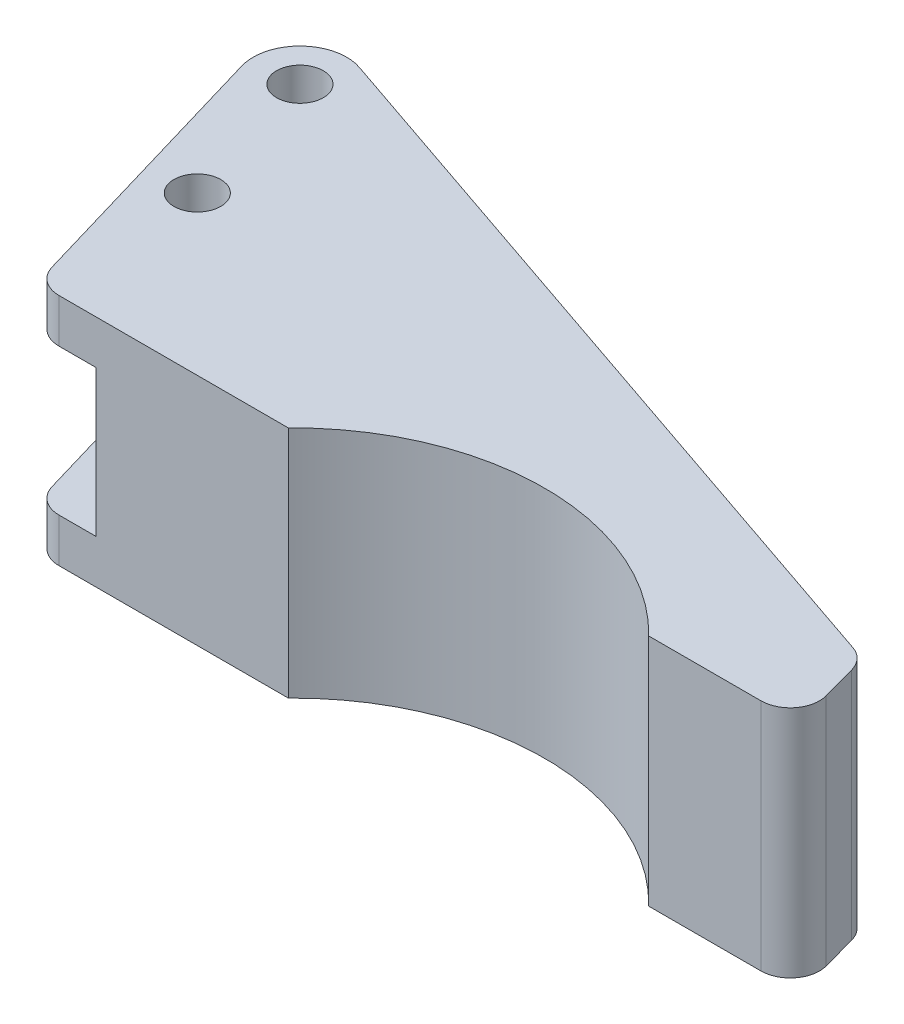
from build123d import *

# Parameters (mm, degrees)
BRACKET_BODY_DEPTH        = 20
MOUNTING_HOLES_SKETCH_R   = 4
MOUNTING_HOLES_2X_8_DEPTH = 20
END_SLOT_SKETCH_W         = 25
END_SLOT_SKETCH_H         = 25
END_SLOT_25_WIDE_DEPTH    = 144.380867308


with BuildPart() as part:
    # Bracket Profile Sketch → Bracket Body (new, symmetric)
    with BuildSketch(Plane(origin=(0, 0, 0), x_dir=(1, 0, 0), z_dir=(0, 1, 0))):
        with BuildLine():
            Line((-1.057217315, 3.586121305), (-14.62477547, 49.607794087))
            ThreePointArc((-14.62477547, 49.607794087), (-12.487512371, 57.644964007), (-4.367320309, 59.441203064))
            Line((-4.367320309, 59.441203064), (123.70369216, 15.732001915))
            ThreePointArc((123.70369216, 15.732001915), (125.729609358, 14.426933511), (126.909739906, 12.325782415))
            Line((126.909739906, 12.325782415), (128.559739906, 6.325782415))
            ThreePointArc((128.559739906, 6.325782415), (127.715452315, 1.969233766), (123.738712942, 0))
            Line((123.738712942, 0), (104.544556544, 0))
            ThreePointArc((104.544556544, 0), (73.738712942, 13), (42.932869341, 0))
            Line((42.932869341, 0), (3.738712942, 0))
            ThreePointArc((3.738712942, 0), (0.744501316, 0.995665256), (-1.057217315, 3.586121305))
        make_face()
    extrude(amount=BRACKET_BODY_DEPTH, both=True)

    # Mounting Holes Sketch → Mounting Holes 2xØ8 (cut, symmetric)
    with BuildSketch(Plane(origin=(0, 0, 0), x_dir=(1, 0, 0), z_dir=(0, 1, 0))):
        with Locations(Location((-6.951287058, 51.87, 0), (0, 0, 270))):
            Circle(MOUNTING_HOLES_SKETCH_R)
        with Locations(Location((0.378712942, 27, 0), (0, 0, 270))):
            Circle(MOUNTING_HOLES_SKETCH_R)
    extrude(amount=MOUNTING_HOLES_2X_8_DEPTH, both=True, mode=Mode.SUBTRACT)

    # End Slot Sketch → End Slot 25 Wide (cut, through all)
    with BuildSketch(Plane.XY):
        with Locations((-2.451287058, 0)):
            Rectangle(END_SLOT_SKETCH_W, END_SLOT_SKETCH_H)
    extrude(amount=-END_SLOT_25_WIDE_DEPTH, mode=Mode.SUBTRACT)


solid = part.part
